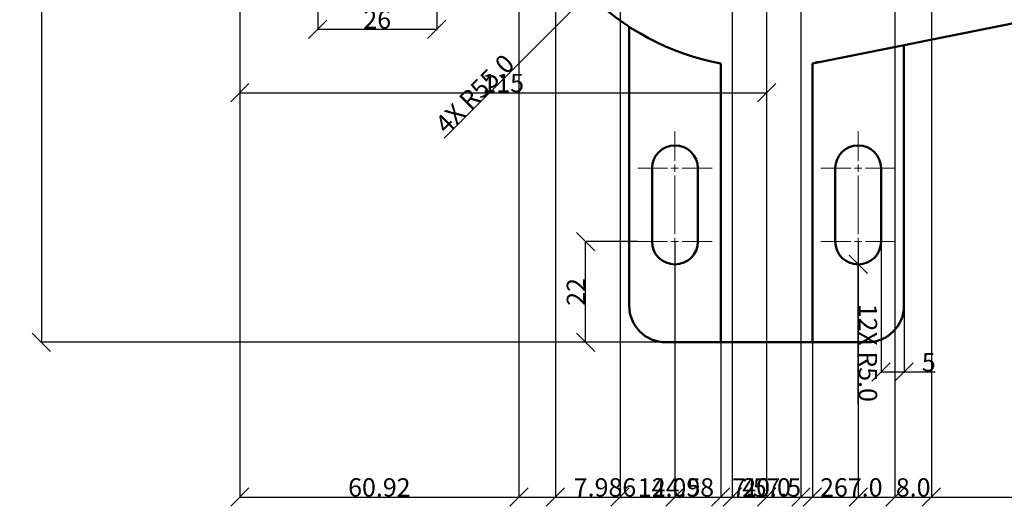
# Model space of a CAD drawing. Units: millimetres. Extents: x 263 to 611, y 50 to 522.
# Tile 1 of 5: x 263 to 478, y 50 to 157. Entities that reach past the tile are written whole.
import ezdxf

# ---------------------------------------------------------------- set-up
doc = ezdxf.new("R2010")
doc.units = ezdxf.units.MM
doc.header["$MEASUREMENT"] = 0
doc.linetypes.add('CENTER', pattern=[50.8, 31.75, -6.35, 6.35, -6.35])
for name, color, linetype, lineweight in [('M-CNTR', 1, 'CENTER', 18), ('M-DIMS', 2, 'Continuous', 25), ('M-OUTL', 7, 'Continuous', 50)]:
    doc.layers.add(name, color=color, linetype=linetype, lineweight=lineweight)
doc.styles.get("Standard").update_dxf_attribs({"font": 'arial.ttf'})
doc.dimstyles.get("Standard").update_dxf_attribs({"dimtxt": 4, "dimasz": 4, "dimexe": 0.18, "dimexo": 0.0625, "dimgap": 0.09, "dimtad": 1, "dimdec": 0, "dimzin": 0, "dimdsep": 46, "dimtxsty": 'Standard', "dimblk": 'OBLIQUE', "dimcen": 0.09, "dimclre": 251, "dimadec": 0, "dimazin": 0, "dimtfac": 1, "dimtdec": 0, "dimtofl": 0, "dimtmove": 0, "dimatfit": 3, "dimfxl": 1, "dimtolj": 1, "dimtzin": 0, "dimarcsym": 0})

# ---------------------------------------------------------------- blocks, each defined once
blk = doc.blocks.new('*U10')
at = {"layer": 'M-CNTR', "color": 0, "transparency": 16777216}
for p, q in [((0, 1.6), (0, 8.12)), ((-8.12, 0), (-1.6, 0)), ((1.6, 0), (8.12, 0)), ((0, -8.12), (0, -1.6))]:
    blk.add_line(p, q, dxfattribs=at)
at = {"layer": 'M-CNTR', "color": 0, "linetype": 'Continuous', "transparency": 16777216}
for p, q in [((-0.8, 0), (0.8, 0)), ((0, -0.8), (0, 0.8))]:
    blk.add_line(p, q, dxfattribs=at)
blk = doc.blocks.new('*U11')
at = {"layer": 'M-CNTR', "color": 0, "transparency": 16777216}
for p, q in [((0, 1.6), (0, 8.12)), ((-8.12, 0), (-1.6, 0)), ((1.6, 0), (8.12, 0)), ((0, -8.12), (0, -1.6))]:
    blk.add_line(p, q, dxfattribs=at)
at = {"layer": 'M-CNTR', "color": 0, "linetype": 'Continuous', "transparency": 16777216}
for p, q in [((-0.8, 0), (0.8, 0)), ((0, -0.8), (0, 0.8))]:
    blk.add_line(p, q, dxfattribs=at)
blk = doc.blocks.new('*U12')
at = {"layer": 'M-CNTR', "color": 0, "transparency": 16777216}
for p, q in [((0, 1.6), (0, 8.12)), ((-8.12, 0), (-1.6, 0)), ((1.6, 0), (8.12, 0)), ((0, -8.12), (0, -1.6))]:
    blk.add_line(p, q, dxfattribs=at)
at = {"layer": 'M-CNTR', "color": 0, "linetype": 'Continuous', "transparency": 16777216}
for p, q in [((-0.8, 0), (0.8, 0)), ((0, -0.8), (0, 0.8))]:
    blk.add_line(p, q, dxfattribs=at)
blk = doc.blocks.new('*U13')
at = {"layer": 'M-CNTR', "color": 0, "transparency": 16777216}
for p, q in [((0, 1.6), (0, 8.12)), ((-8.12, 0), (-1.6, 0)), ((1.6, 0), (8.12, 0)), ((0, -8.12), (0, -1.6))]:
    blk.add_line(p, q, dxfattribs=at)
at = {"layer": 'M-CNTR', "color": 0, "linetype": 'Continuous', "transparency": 16777216}
for p, q in [((-0.8, 0), (0.8, 0)), ((0, -0.8), (0, 0.8))]:
    blk.add_line(p, q, dxfattribs=at)
blk = doc.blocks.new('_Oblique')
at = {"color": 0, "linetype": 'ByBlock', "lineweight": -2}
blk.add_line((-0.5, -0.5), (0.5, 0.5), dxfattribs=at)
blk = doc.blocks.new('*D22')
at = {"layer": 'Defpoints', "color": 0, "transparency": 16777216}
for p in [(404.1, 316.08), (267.8, 86.08), (404.1, 86.08)]:
    blk.add_point(p, dxfattribs=at)
at = {"layer": 'M-DIMS', "color": 0, "lineweight": -2, "transparency": 16777216}
for p, q in [((404.04, 316.08), (267.62, 316.08)), ((267.8, 316.08), (267.8, 86.08)), ((404.04, 86.08), (267.62, 86.08))]:
    blk.add_line(p, q, dxfattribs=at)
at = {"layer": 'M-DIMS', "color": 0, "lineweight": -2, "transparency": 16777216, "xscale": 4, "yscale": 4, "zscale": 4}
for p, rotation in [((267.8, 316.08), 90), ((267.8, 86.08), 270)]:
    blk.add_blockref('_Oblique', p, dxfattribs=dict(at, rotation=rotation))
at = {"layer": 'M-DIMS', "color": 0, "transparency": 16777216, "insert": (265.67, 201.08), "char_height": 4, "attachment_point": 5, "rotation": 90}
blk.add_mtext('\\A1;230', dxfattribs=at)
blk = doc.blocks.new('*D24')
at = {"layer": 'Defpoints', "color": 0, "transparency": 16777216}
for p in [(328.1, 181.08), (354.1, 181.08), (354.1, 154.45)]:
    blk.add_point(p, dxfattribs=at)
at = {"layer": 'M-DIMS', "color": 0, "lineweight": -2, "transparency": 16777216}
for p, q in [((328.1, 181.02), (328.1, 154.27)), ((354.1, 181.02), (354.1, 154.27)), ((328.1, 154.45), (354.1, 154.45))]:
    blk.add_line(p, q, dxfattribs=at)
at = {"layer": 'M-DIMS', "color": 0, "lineweight": -2, "transparency": 16777216, "xscale": 4, "yscale": 4, "zscale": 4, "rotation": 180}
blk.add_blockref('_Oblique', (328.1, 154.45), dxfattribs=at)
at = {"layer": 'M-DIMS', "color": 0, "lineweight": -2, "transparency": 16777216, "xscale": 4, "yscale": 4, "zscale": 4}
blk.add_blockref('_Oblique', (354.1, 154.45), dxfattribs=at)
at = {"layer": 'M-DIMS', "color": 0, "transparency": 16777216, "insert": (341.1, 156.58), "char_height": 4, "attachment_point": 5}
blk.add_mtext('\\A1;26', dxfattribs=at)
blk = doc.blocks.new('*D25')
at = {"layer": 'Defpoints', "color": 0, "transparency": 16777216}
for p in [(311.1, 201.08), (426.1, 201.08), (426.1, 140.57)]:
    blk.add_point(p, dxfattribs=at)
at = {"layer": 'M-DIMS', "color": 0, "lineweight": -2, "transparency": 16777216}
for p, q in [((311.1, 201.02), (311.1, 140.39)), ((426.1, 201.02), (426.1, 140.39)), ((311.1, 140.57), (426.1, 140.57))]:
    blk.add_line(p, q, dxfattribs=at)
at = {"layer": 'M-DIMS', "color": 0, "lineweight": -2, "transparency": 16777216, "xscale": 4, "yscale": 4, "zscale": 4, "rotation": 180}
blk.add_blockref('_Oblique', (311.1, 140.57), dxfattribs=at)
at = {"layer": 'M-DIMS', "color": 0, "lineweight": -2, "transparency": 16777216, "xscale": 4, "yscale": 4, "zscale": 4}
blk.add_blockref('_Oblique', (426.1, 140.57), dxfattribs=at)
at = {"layer": 'M-DIMS', "color": 0, "transparency": 16777216, "insert": (368.6, 142.7), "char_height": 4, "attachment_point": 5}
blk.add_mtext('\\A1;115', dxfattribs=at)
blk = doc.blocks.new('*D27')
at = {"layer": 'Defpoints', "color": 0, "transparency": 16777216}
for p in [(386.57, 108.08), (397.98, 108.08), (404.1, 86.08)]:
    blk.add_point(p, dxfattribs=at)
at = {"layer": 'M-DIMS', "color": 0, "lineweight": -2, "transparency": 16777216}
for p, q in [((397.92, 108.08), (386.39, 108.08)), ((386.57, 86.08), (386.57, 108.08)), ((404.04, 86.08), (386.39, 86.08))]:
    blk.add_line(p, q, dxfattribs=at)
at = {"layer": 'M-DIMS', "color": 0, "lineweight": -2, "transparency": 16777216, "xscale": 4, "yscale": 4, "zscale": 4}
for p, rotation in [((386.57, 108.08), 90), ((386.57, 86.08), 270)]:
    blk.add_blockref('_Oblique', p, dxfattribs=dict(at, rotation=rotation))
at = {"layer": 'M-DIMS', "color": 0, "transparency": 16777216, "insert": (384.47, 97.08), "char_height": 4, "attachment_point": 5, "rotation": 90}
blk.add_mtext('\\A1;22', dxfattribs=at)
blk = doc.blocks.new('*D36')
at = {"layer": 'Defpoints', "color": 0, "transparency": 16777216}
for p in [(451.1, 108.08), (456.1, 94.08), (451.1, 79.59)]:
    blk.add_point(p, dxfattribs=at)
at = {"layer": 'M-DIMS', "color": 0, "lineweight": -2, "transparency": 16777216}
for p, q in [((451.1, 108.02), (451.1, 79.41)), ((456.1, 94.02), (456.1, 79.41)), ((451.1, 79.59), (456.1, 79.59)), ((456.1, 79.59), (462.93, 79.59))]:
    blk.add_line(p, q, dxfattribs=at)
at = {"layer": 'M-DIMS', "color": 0, "lineweight": -2, "transparency": 16777216, "xscale": 4, "yscale": 4, "zscale": 4, "rotation": 180}
blk.add_blockref('_Oblique', (451.1, 79.59), dxfattribs=at)
at = {"layer": 'M-DIMS', "color": 0, "lineweight": -2, "transparency": 16777216, "xscale": 4, "yscale": 4, "zscale": 4}
blk.add_blockref('_Oblique', (456.1, 79.59), dxfattribs=at)
at = {"layer": 'M-DIMS', "color": 0, "transparency": 16777216, "insert": (461.51, 81.71), "char_height": 4, "attachment_point": 5}
blk.add_mtext('\\A1;5', dxfattribs=at)
blk = doc.blocks.new('SLOT-10x26')
for p, q in [((0, 5), (0, 21)), ((10, 5), (10, 21))]:
    blk.add_line(p, q)
for centre, start, end in [((5, 21), 0, 180), ((5, 5), 180, 0)]:
    blk.add_arc(centre, 5, start, end)
blk = doc.blocks.new('*D50')
at = {"layer": 'Defpoints', "color": 0, "transparency": 16777216}
for p in [(416.1, 86.08), (436.1, 86.08), (436.1, 52.26)]:
    blk.add_point(p, dxfattribs=at)
at = {"layer": 'M-DIMS', "color": 251, "lineweight": -2, "transparency": 16777216}
for p, q in [((416.1, 86.02), (416.1, 52.08)), ((436.1, 86.02), (436.1, 52.08))]:
    blk.add_line(p, q, dxfattribs=at)
at = {"layer": 'M-DIMS', "color": 0, "lineweight": -2, "transparency": 16777216}
blk.add_line((416.1, 52.26), (436.1, 52.26), dxfattribs=at)
at = {"layer": 'M-DIMS', "color": 0, "lineweight": -2, "transparency": 16777216, "xscale": 4, "yscale": 4, "zscale": 4, "rotation": 180}
blk.add_blockref('_Oblique', (416.1, 52.26), dxfattribs=at)
at = {"layer": 'M-DIMS', "color": 0, "lineweight": -2, "transparency": 16777216, "xscale": 4, "yscale": 4, "zscale": 4}
blk.add_blockref('_Oblique', (436.1, 52.26), dxfattribs=at)
at = {"layer": 'M-DIMS', "color": 0, "transparency": 16777216, "insert": (426.1, 54.39), "char_height": 4, "attachment_point": 5}
blk.add_mtext('\\A1;20.0', dxfattribs=at)
blk = doc.blocks.new('*D51')
at = {"layer": 'Defpoints', "color": 0, "transparency": 16777216}
for p in [(406.1, 108.08), (446.1, 108.08), (446.1, 52.26)]:
    blk.add_point(p, dxfattribs=at)
at = {"layer": 'M-DIMS', "color": 251, "lineweight": -2, "transparency": 16777216}
for p, q in [((406.1, 108.02), (406.1, 52.08)), ((446.1, 108.02), (446.1, 52.08))]:
    blk.add_line(p, q, dxfattribs=at)
at = {"layer": 'M-DIMS', "color": 0, "lineweight": -2, "transparency": 16777216}
blk.add_line((406.1, 52.26), (446.1, 52.26), dxfattribs=at)
at = {"layer": 'M-DIMS', "color": 0, "lineweight": -2, "transparency": 16777216, "xscale": 4, "yscale": 4, "zscale": 4, "rotation": 180}
blk.add_blockref('_Oblique', (406.1, 52.26), dxfattribs=at)
at = {"layer": 'M-DIMS', "color": 0, "lineweight": -2, "transparency": 16777216, "xscale": 4, "yscale": 4, "zscale": 4}
blk.add_blockref('_Oblique', (446.1, 52.26), dxfattribs=at)
at = {"layer": 'M-DIMS', "color": 0, "transparency": 16777216, "insert": (426.1, 54.39), "char_height": 4, "attachment_point": 5}
blk.add_mtext('\\A1;40.0', dxfattribs=at)
blk = doc.blocks.new('*D53')
at = {"layer": 'Defpoints', "color": 0, "transparency": 16777216}
for p in [(578.1, 423.27), (311.1, 383.27), (578.1, 52.26)]:
    blk.add_point(p, dxfattribs=at)
at = {"layer": 'M-DIMS', "color": 251, "lineweight": -2, "transparency": 16777216}
for p, q in [((578.1, 423.21), (578.1, 52.08)), ((311.1, 383.21), (311.1, 52.08))]:
    blk.add_line(p, q, dxfattribs=at)
at = {"layer": 'M-DIMS', "color": 0, "lineweight": -2, "transparency": 16777216}
blk.add_line((311.1, 52.26), (578.1, 52.26), dxfattribs=at)
at = {"layer": 'M-DIMS', "color": 0, "lineweight": -2, "transparency": 16777216, "xscale": 4, "yscale": 4, "zscale": 4, "rotation": 180}
blk.add_blockref('_Oblique', (311.1, 52.26), dxfattribs=at)
at = {"layer": 'M-DIMS', "color": 0, "lineweight": -2, "transparency": 16777216, "xscale": 4, "yscale": 4, "zscale": 4}
blk.add_blockref('_Oblique', (578.1, 52.26), dxfattribs=at)
at = {"layer": 'M-DIMS', "color": 0, "transparency": 16777216, "insert": (444.6, 54.39), "char_height": 4, "attachment_point": 5}
blk.add_mtext('\\A1;267.0', dxfattribs=at)
blk = doc.blocks.new('*D56')
at = {"layer": 'Defpoints', "color": 0, "transparency": 16777216}
for p in [(454.1, 410.27), (462.1, 410.27), (462.1, 52.26)]:
    blk.add_point(p, dxfattribs=at)
at = {"layer": 'M-DIMS', "color": 251, "lineweight": -2, "transparency": 16777216}
for p, q in [((454.1, 410.21), (454.1, 52.08)), ((462.1, 410.21), (462.1, 52.08))]:
    blk.add_line(p, q, dxfattribs=at)
at = {"layer": 'M-DIMS', "color": 0, "lineweight": -2, "transparency": 16777216}
blk.add_line((454.1, 52.26), (462.1, 52.26), dxfattribs=at)
at = {"layer": 'M-DIMS', "color": 0, "lineweight": -2, "transparency": 16777216, "xscale": 4, "yscale": 4, "zscale": 4, "rotation": 180}
blk.add_blockref('_Oblique', (454.1, 52.26), dxfattribs=at)
at = {"layer": 'M-DIMS', "color": 0, "lineweight": -2, "transparency": 16777216, "xscale": 4, "yscale": 4, "zscale": 4}
blk.add_blockref('_Oblique', (462.1, 52.26), dxfattribs=at)
at = {"layer": 'M-DIMS', "color": 0, "transparency": 16777216, "insert": (458.1, 54.39), "char_height": 4, "attachment_point": 5}
blk.add_mtext('\\A1;8.0', dxfattribs=at)
blk = doc.blocks.new('*D57')
at = {"layer": 'Defpoints', "color": 0, "transparency": 16777216}
for p in [(372.02, 403.27), (311.1, 383.27), (372.02, 52.26)]:
    blk.add_point(p, dxfattribs=at)
at = {"layer": 'M-DIMS', "color": 251, "lineweight": -2, "transparency": 16777216}
for p, q in [((372.02, 403.21), (372.02, 52.08)), ((311.1, 383.21), (311.1, 52.08))]:
    blk.add_line(p, q, dxfattribs=at)
at = {"layer": 'M-DIMS', "color": 0, "lineweight": -2, "transparency": 16777216}
blk.add_line((311.1, 52.26), (372.02, 52.26), dxfattribs=at)
at = {"layer": 'M-DIMS', "color": 0, "lineweight": -2, "transparency": 16777216, "xscale": 4, "yscale": 4, "zscale": 4, "rotation": 180}
blk.add_blockref('_Oblique', (311.1, 52.26), dxfattribs=at)
at = {"layer": 'M-DIMS', "color": 0, "lineweight": -2, "transparency": 16777216, "xscale": 4, "yscale": 4, "zscale": 4}
blk.add_blockref('_Oblique', (372.02, 52.26), dxfattribs=at)
at = {"layer": 'M-DIMS', "color": 0, "transparency": 16777216, "insert": (341.56, 54.39), "char_height": 4, "attachment_point": 5}
blk.add_mtext('\\A1;60.92', dxfattribs=at)
blk = doc.blocks.new('*D58')
at = {"layer": 'Defpoints', "color": 0, "transparency": 16777216}
for p in [(372.02, 403.27), (380, 383.27), (380, 52.26)]:
    blk.add_point(p, dxfattribs=at)
at = {"layer": 'M-DIMS', "color": 251, "lineweight": -2, "transparency": 16777216}
for p, q in [((372.02, 403.21), (372.02, 52.08)), ((380, 383.21), (380, 52.08))]:
    blk.add_line(p, q, dxfattribs=at)
at = {"layer": 'M-DIMS', "color": 0, "lineweight": -2, "transparency": 16777216}
for p, q in [((372.02, 52.26), (380, 52.26)), ((380, 52.26), (397.64, 52.26))]:
    blk.add_line(p, q, dxfattribs=at)
at = {"layer": 'M-DIMS', "color": 0, "lineweight": -2, "transparency": 16777216, "xscale": 4, "yscale": 4, "zscale": 4, "rotation": 180}
blk.add_blockref('_Oblique', (372.02, 52.26), dxfattribs=at)
at = {"layer": 'M-DIMS', "color": 0, "lineweight": -2, "transparency": 16777216, "xscale": 4, "yscale": 4, "zscale": 4}
blk.add_blockref('_Oblique', (380, 52.26), dxfattribs=at)
at = {"layer": 'M-DIMS', "color": 0, "transparency": 16777216, "insert": (390.82, 54.39), "char_height": 4, "attachment_point": 5}
blk.add_mtext('\\A1;7.986', dxfattribs=at)
blk = doc.blocks.new('*D59')
at = {"layer": 'Defpoints', "color": 0, "transparency": 16777216}
for p in [(380, 383.27), (394.1, 383.27), (394.1, 52.26)]:
    blk.add_point(p, dxfattribs=at)
at = {"layer": 'M-DIMS', "color": 251, "lineweight": -2, "transparency": 16777216}
for p, q in [((380, 383.21), (380, 52.08)), ((394.1, 383.21), (394.1, 52.08))]:
    blk.add_line(p, q, dxfattribs=at)
at = {"layer": 'M-DIMS', "color": 0, "lineweight": -2, "transparency": 16777216}
for p, q in [((380, 52.26), (394.1, 52.26)), ((394.1, 52.26), (414.52, 52.26))]:
    blk.add_line(p, q, dxfattribs=at)
at = {"layer": 'M-DIMS', "color": 0, "lineweight": -2, "transparency": 16777216, "xscale": 4, "yscale": 4, "zscale": 4, "rotation": 180}
blk.add_blockref('_Oblique', (380, 52.26), dxfattribs=at)
at = {"layer": 'M-DIMS', "color": 0, "lineweight": -2, "transparency": 16777216, "xscale": 4, "yscale": 4, "zscale": 4}
blk.add_blockref('_Oblique', (394.1, 52.26), dxfattribs=at)
at = {"layer": 'M-DIMS', "color": 0, "transparency": 16777216, "insert": (406.31, 54.39), "char_height": 4, "attachment_point": 5}
blk.add_mtext('\\A1;14.098', dxfattribs=at)
blk = doc.blocks.new('*D60')
at = {"layer": 'Defpoints', "color": 0, "transparency": 16777216}
for p in [(418.6, 403.27), (394.1, 383.27), (418.6, 52.26)]:
    blk.add_point(p, dxfattribs=at)
at = {"layer": 'M-DIMS', "color": 251, "lineweight": -2, "transparency": 16777216}
for p, q in [((418.6, 403.21), (418.6, 52.08)), ((394.1, 383.21), (394.1, 52.08))]:
    blk.add_line(p, q, dxfattribs=at)
at = {"layer": 'M-DIMS', "color": 0, "lineweight": -2, "transparency": 16777216}
blk.add_line((394.1, 52.26), (418.6, 52.26), dxfattribs=at)
at = {"layer": 'M-DIMS', "color": 0, "lineweight": -2, "transparency": 16777216, "xscale": 4, "yscale": 4, "zscale": 4, "rotation": 180}
blk.add_blockref('_Oblique', (394.1, 52.26), dxfattribs=at)
at = {"layer": 'M-DIMS', "color": 0, "lineweight": -2, "transparency": 16777216, "xscale": 4, "yscale": 4, "zscale": 4}
blk.add_blockref('_Oblique', (418.6, 52.26), dxfattribs=at)
at = {"layer": 'M-DIMS', "color": 0, "transparency": 16777216, "insert": (406.35, 54.39), "char_height": 4, "attachment_point": 5}
blk.add_mtext('\\A1;24.5', dxfattribs=at)
blk = doc.blocks.new('*D61')
at = {"layer": 'Defpoints', "color": 0, "transparency": 16777216}
for p in [(418.6, 403.27), (426.1, 378.63), (426.1, 52.26)]:
    blk.add_point(p, dxfattribs=at)
at = {"layer": 'M-DIMS', "color": 251, "lineweight": -2, "transparency": 16777216}
for p, q in [((418.6, 403.21), (418.6, 52.08)), ((426.1, 378.57), (426.1, 52.08))]:
    blk.add_line(p, q, dxfattribs=at)
at = {"layer": 'M-DIMS', "color": 0, "lineweight": -2, "transparency": 16777216}
blk.add_line((418.6, 52.26), (426.1, 52.26), dxfattribs=at)
at = {"layer": 'M-DIMS', "color": 0, "lineweight": -2, "transparency": 16777216, "xscale": 4, "yscale": 4, "zscale": 4, "rotation": 180}
blk.add_blockref('_Oblique', (418.6, 52.26), dxfattribs=at)
at = {"layer": 'M-DIMS', "color": 0, "lineweight": -2, "transparency": 16777216, "xscale": 4, "yscale": 4, "zscale": 4}
blk.add_blockref('_Oblique', (426.1, 52.26), dxfattribs=at)
at = {"layer": 'M-DIMS', "color": 0, "transparency": 16777216, "insert": (422.35, 54.38), "char_height": 4, "attachment_point": 5}
blk.add_mtext('\\A1;7.5', dxfattribs=at)
blk = doc.blocks.new('*D62')
at = {"layer": 'Defpoints', "color": 0, "transparency": 16777216}
for p in [(433.6, 383.27), (426.1, 378.63), (433.6, 52.26)]:
    blk.add_point(p, dxfattribs=at)
at = {"layer": 'M-DIMS', "color": 251, "lineweight": -2, "transparency": 16777216}
for p, q in [((433.6, 383.21), (433.6, 52.08)), ((426.1, 378.57), (426.1, 52.08))]:
    blk.add_line(p, q, dxfattribs=at)
at = {"layer": 'M-DIMS', "color": 0, "lineweight": -2, "transparency": 16777216}
blk.add_line((426.1, 52.26), (433.6, 52.26), dxfattribs=at)
at = {"layer": 'M-DIMS', "color": 0, "lineweight": -2, "transparency": 16777216, "xscale": 4, "yscale": 4, "zscale": 4, "rotation": 180}
blk.add_blockref('_Oblique', (426.1, 52.26), dxfattribs=at)
at = {"layer": 'M-DIMS', "color": 0, "lineweight": -2, "transparency": 16777216, "xscale": 4, "yscale": 4, "zscale": 4}
blk.add_blockref('_Oblique', (433.6, 52.26), dxfattribs=at)
at = {"layer": 'M-DIMS', "color": 0, "transparency": 16777216, "insert": (429.85, 54.38), "char_height": 4, "attachment_point": 5}
blk.add_mtext('\\A1;7.5', dxfattribs=at)
blk = doc.blocks.new('*D69')
at = {"layer": 'Defpoints', "color": 0, "transparency": 16777216}
for p in [(426.1, 201.08), (387.21, 162.19)]:
    blk.add_point(p, dxfattribs=at)
at = {"layer": 'M-DIMS', "color": 251, "lineweight": -2, "transparency": 16777216}
for p, q in [((426.01, 201.08), (426.19, 201.08)), ((426.1, 200.99), (426.1, 201.17))]:
    blk.add_line(p, q, dxfattribs=at)
at = {"layer": 'M-DIMS', "color": 0, "lineweight": -2, "transparency": 16777216}
blk.add_line((355.69, 130.68), (387.21, 162.19), dxfattribs=at)
at = {"layer": 'M-DIMS', "color": 0, "lineweight": -2, "transparency": 16777216, "xscale": 4, "yscale": 4, "zscale": 4, "rotation": 44.99977533015295}
blk.add_blockref('_Oblique', (387.21, 162.19), dxfattribs=at)
at = {"layer": 'M-DIMS', "color": 0, "transparency": 16777216, "insert": (362.37, 140.36), "char_height": 4, "attachment_point": 5, "rotation": 44.9998}
blk.add_mtext('\\A1;4X R55.0', dxfattribs=at)
blk = doc.blocks.new('*D81')
at = {"layer": 'Defpoints', "color": 0, "transparency": 16777216}
for p in [(446.1, 108.08), (446.1, 103.08)]:
    blk.add_point(p, dxfattribs=at)
at = {"layer": 'M-DIMS', "color": 251, "lineweight": -2, "transparency": 16777216}
for p, q in [((446.01, 108.08), (446.19, 108.08)), ((446.1, 107.99), (446.1, 108.17))]:
    blk.add_line(p, q, dxfattribs=at)
at = {"layer": 'M-DIMS', "color": 0, "lineweight": -2, "transparency": 16777216}
blk.add_line((446.1, 72.48), (446.1, 103.08), dxfattribs=at)
at = {"layer": 'M-DIMS', "color": 0, "lineweight": -2, "transparency": 16777216, "xscale": 4, "yscale": 4, "zscale": 4, "rotation": 90.00189076072301}
blk.add_blockref('_Oblique', (446.1, 103.08), dxfattribs=at)
at = {"layer": 'M-DIMS', "color": 0, "transparency": 16777216, "insert": (448.23, 83.78), "char_height": 4, "attachment_point": 5, "rotation": 270.0019}
blk.add_mtext('\\A1;12X R5.0', dxfattribs=at)

msp = doc.modelspace()

# ---------------------------------------------------------------- linework, layer by layer
at = {"layer": 'M-CNTR'}
msp.add_line((426.0988, 323.9478), (426.0988, 74.3557), dxfattribs=at)
at = {"layer": 'M-OUTL'}
for p, q in [((552.2661, 170.1912), (436.0988, 146.9983)), ((396.0988, 94.0815), (396.0988, 154.9838)), ((456.0988, 94.0815), (456.0988, 150.9913)), ((416.0988, 86.0815), (416.0988, 146.9983)), ((436.0988, 86.0815), (436.0988, 146.9983)), ((448.0988, 86.0815), (404.0988, 86.0815))]:
    msp.add_line(p, q, dxfattribs=at)
for centre, radius, start, end in [((426.0988, 201.0815), 55, 190.475682, 259.524318), ((426.0988, 201.0815), 55, 280.475682, 282.105717), ((404.0988, 94.0815), 8, 180, 270), ((448.0988, 94.0815), 8, 270, 0)]:
    msp.add_arc(centre, radius, start, end, dxfattribs=at)

# ---------------------------------------------------------------- block references
at = {"layer": 'M-CNTR'}
for name, p in [('*U10', (406.0988, 124.0815)), ('*U12', (446.0988, 124.0815)), ('*U11', (406.0988, 108.0815)), ('*U13', (446.0988, 108.0815))]:
    msp.add_blockref(name, p, dxfattribs=at)
at = {"layer": 'M-OUTL', "rotation": 180}
msp.add_blockref('SLOT-10x26', (411.0987, 129.0811), dxfattribs=at)
at = {"layer": 'M-OUTL'}
msp.add_blockref('SLOT-10x26', (441.099, 103.082), dxfattribs=at)

# ---------------------------------------------------------------- dimensions: what is measured, and where the dimension line sits
at = {"layer": 'M-DIMS'}
for base, p1, p2, override, picture, middle in [((578.0988, 52.2557), (311.0988, 383.2727), (578.0988, 423.2727), {"dimdec": 1, "dimlfac": 1, "dimrnd": 0, "dimzin": 0, "dimdsep": 46, "dimlunit": 2}, '*D53', (444.5988, 54.388)), ((462.0988, 52.2557), (454.0988, 410.2727), (462.0988, 410.2727), {"dimdec": 1, "dimlfac": 1, "dimrnd": 0, "dimzin": 0, "dimdsep": 46, "dimlunit": 2}, '*D56', (458.0988, 54.388)), ((372.0156, 52.2557), (311.0988, 383.2727), (372.0156, 403.2727), {"dimdec": 2, "dimlfac": 1, "dimrnd": 0, "dimzin": 0, "dimdsep": 46, "dimlunit": 2}, '*D57', (341.5572, 54.388)), ((380.00111, 52.25572), (372.01556, 403.2727), (380.00111, 383.2727), {"dimdec": 3, "dimlfac": 1, "dimrnd": 0, "dimzin": 0, "dimdsep": 46, "dimlunit": 2}, '*D58', (390.82235, 54.38801)), ((418.5988, 52.2557), (394.0988, 383.2727), (418.5988, 403.2727), {"dimdec": 1, "dimlfac": 1, "dimrnd": 0, "dimzin": 0, "dimdsep": 46, "dimlunit": 2}, '*D60', (406.3488, 54.388)), ((426.0988, 52.2557), (418.5988, 403.2727), (426.0988, 378.6323), {"dimdec": 1, "dimlfac": 1, "dimrnd": 0, "dimzin": 0, "dimdsep": 46, "dimlunit": 2}, '*D61', (422.3488, 54.3798)), ((394.0988, 52.2557), (380.0011, 383.2727), (394.0988, 383.2727), {"dimdec": 3, "dimlfac": 1, "dimrnd": 0, "dimzin": 0, "dimdsep": 46, "dimlunit": 2}, '*D59', (406.3075, 54.388)), ((433.5988, 52.2557), (426.0988, 378.6323), (433.5988, 383.2727), {"dimdec": 1, "dimlfac": 1, "dimrnd": 0, "dimzin": 0, "dimdsep": 46, "dimlunit": 2}, '*D62', (429.8488, 54.3798)), ((426.0988, 140.5664), (311.0988, 201.0815), (426.0988, 201.0815), {"dimclrd": 0, "dimclre": 0, "dimclrt": 0}, '*D25', (368.5988, 142.6987)), ((354.0988, 154.4515), (328.0988, 181.0815), (354.0988, 181.0815), {"dimclrd": 0, "dimclre": 0, "dimclrt": 0}, '*D24', (341.0988, 156.5838)), ((446.0988, 52.2557), (406.0988, 108.0815), (446.0988, 108.0815), {"dimdec": 1, "dimlfac": 1, "dimrnd": 0, "dimzin": 0, "dimdsep": 46, "dimlunit": 2}, '*D51', (426.0988, 54.388)), ((436.0988, 52.2557), (416.0988, 86.0815), (436.0988, 86.0815), {"dimdec": 1, "dimlfac": 1, "dimrnd": 0, "dimzin": 0, "dimdsep": 46, "dimlunit": 2}, '*D50', (426.0988, 54.388))]:
    dim = msp.add_linear_dim(base=base, p1=p1, p2=p2, dimstyle='Standard', override=override, dxfattribs=at)
    dim.commit()
    dim.dimension.update_dxf_attribs({"geometry": picture, "text_midpoint": middle})
for base, p1, p2, picture, middle in [((267.7992, 86.0815), (404.0988, 316.0815), (404.0988, 86.0815), '*D22', (265.6656, 201.0815)), ((386.572, 108.0815), (404.0988, 86.0815), (397.9788, 108.0815), '*D27', (384.4738, 97.0815))]:
    dim = msp.add_linear_dim(base=base, p1=p1, p2=p2, angle=90, dimstyle='Standard', override={"dimclrd": 0, "dimclre": 0, "dimclrt": 0}, dxfattribs=at)
    dim.commit()
    dim.dimension.update_dxf_attribs({"geometry": picture, "text_midpoint": middle})
dim = msp.add_radius_dim(center=(426.0988, 201.0815), mpoint=(387.2078, 162.1908), text='4X <>', dimstyle='Standard', override={"dimdec": 1, "dimlfac": 1, "dimrnd": 0, "dimzin": 0, "dimdsep": 46, "dimlunit": 2}, dxfattribs=at)
dim.commit()
dim.dimension.update_dxf_attribs({"geometry": '*D69', "text_midpoint": (363.8732, 138.8564), "dimtype": 164})
dim = msp.add_radius_dim(center=(446.0988, 108.0815), mpoint=(446.099, 103.0815), text='12X <>', dimstyle='Standard', override={"dimdec": 1, "dimlfac": 1, "dimrnd": 0, "dimzin": 0, "dimdsep": 46, "dimlunit": 2}, dxfattribs=at)
dim.commit()
dim.dimension.update_dxf_attribs({"geometry": '*D81', "text_midpoint": (448.2319, 83.7801)})
dim = msp.add_linear_dim(base=(451.0988, 79.586), p1=(456.0988, 94.0815), p2=(451.0988, 108.0815), dimstyle='Standard', override={"dimclrd": 0, "dimclre": 0, "dimclrt": 0}, dxfattribs=at)
dim.commit()
dim.dimension.update_dxf_attribs({"geometry": '*D36', "text_midpoint": (461.5149, 79.586), "dimtype": 160})

doc.saveas('drawing.dxf')
